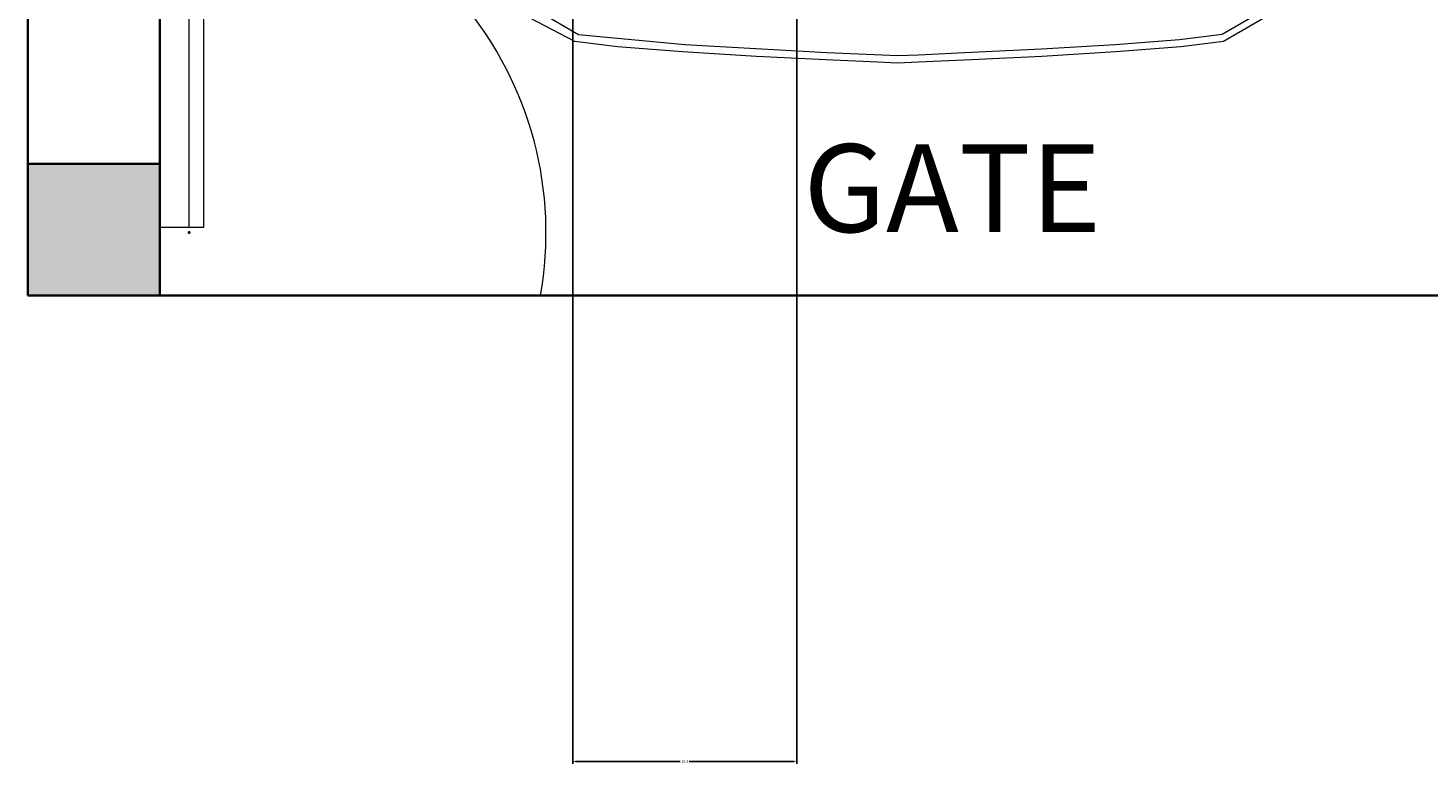
# Model space of a CAD drawing. Units: inches. Extents: x 5 to 421, y -617 to 43.
# Tile 1 of 15: x 37 to 133, y -617 to -566. Entities that reach past the tile are written whole.
import ezdxf

# ---------------------------------------------------------------- set-up
doc = ezdxf.new("R2010")
doc.units = ezdxf.units.IN
doc.header["$MEASUREMENT"] = 0
for name, color, linetype, lineweight in [('A-ANNO-DIMS', 2, 'Continuous', 18), ('A-ANNO-TEXT', 7, 'Continuous', 18), ('A-SITE-GATE', 3, 'Continuous', 20), ('A-SITE-VEHC', 8, 'Continuous', 13), ('A-WALL', 7, 'Continuous', 35)]:
    doc.layers.add(name, color=color, linetype=linetype, lineweight=lineweight)
doc.layers.add('A-WALL-PATT', color=251, linetype='Continuous', lineweight=13, true_color=0x636466)
doc.styles.get("Standard").update_dxf_attribs({"font": 'arial.ttf'})
doc.dimstyles.get("Standard").update_dxf_attribs({"dimtxt": 0.18, "dimasz": 0.18, "dimexe": 0.18, "dimexo": 0.0625, "dimgap": 0.09, "dimtad": 0, "dimtih": 1, "dimtoh": 1, "dimdec": 0, "dimzin": 0, "dimdsep": 46, "dimlunit": 3, "dimtxsty": 'Standard', "dimcen": 0.09, "dimadec": 0, "dimazin": 0, "dimtfac": 1, "dimtdec": 0, "dimtofl": 0, "dimtmove": 0, "dimatfit": 3, "dimfxl": 1, "dimtolj": 1, "dimtzin": 0, "dimarcsym": 0})

# ---------------------------------------------------------------- blocks, each defined once
blk = doc.blocks.new('*D78')
at = {"layer": 'A-ANNO-DIMS', "color": 0, "lineweight": -2, "transparency": 16777216}
for p, q in [((74.624, -338.19), (74.624, -616.599)), ((89.924, -338.331), (89.924, -616.599)), ((74.804, -616.419), (81.958, -616.419)), ((89.744, -616.419), (82.589, -616.419))]:
    blk.add_line(p, q, dxfattribs=at)
at = {"layer": 'A-ANNO-DIMS', "color": 0, "transparency": 16777216}
for points in [[(74.804, -616.389), (74.804, -616.449), (74.624, -616.419)], [(89.744, -616.389), (89.744, -616.449), (89.924, -616.419)]]:
    blk.add_solid(points, dxfattribs=at)
at = {"layer": 'Defpoints', "color": 0, "transparency": 16777216}
for p in [(74.624, -338.127), (89.924, -338.269), (89.924, -616.419)]:
    blk.add_point(p, dxfattribs=at)
at = {"layer": 'A-ANNO-DIMS', "color": 0, "transparency": 16777216, "insert": (82.274, -616.419), "char_height": 0.18, "attachment_point": 5}
blk.add_mtext('\\A1;15.3', dxfattribs=at)
blk = doc.blocks.new('*D81')
at = {"layer": 'A-ANNO-DIMS', "color": 0, "lineweight": -2, "transparency": 16777216}
for p, q in [((78.334, -555.287), (67.254, -564.56)), ((78.514, -555.287), (78.334, -555.287)), ((48.33, -580.324), (48.51, -580.324)), ((48.42, -580.414), (48.42, -580.234))]:
    blk.add_line(p, q, dxfattribs=at)
at = {"layer": 'A-ANNO-DIMS', "color": 0, "transparency": 16777216}
blk.add_solid([(67.235, -564.537), (67.274, -564.583), (67.116, -564.676)], dxfattribs=at)
at = {"layer": 'Defpoints', "color": 0, "transparency": 16777216}
for p in [(67.116, -564.676), (48.42, -580.324)]:
    blk.add_point(p, dxfattribs=at)
at = {"layer": 'A-ANNO-DIMS', "color": 0, "transparency": 16777216, "insert": (78.994, -555.287), "char_height": 0.18, "attachment_point": 5}
blk.add_mtext('\\A1;R24.38', dxfattribs=at)
blk = doc.blocks.new('*D82')
at = {"layer": 'A-ANNO-DIMS', "color": 0, "lineweight": -2, "transparency": 16777216}
for p, q in [((128.083, -555.094), (128.263, -555.094)), ((128.263, -555.094), (139.433, -564.316)), ((158.33, -579.992), (158.51, -579.992)), ((158.42, -580.082), (158.42, -579.902))]:
    blk.add_line(p, q, dxfattribs=at)
at = {"layer": 'A-ANNO-DIMS', "color": 0, "transparency": 16777216}
blk.add_solid([(139.452, -564.293), (139.414, -564.339), (139.572, -564.431)], dxfattribs=at)
at = {"layer": 'Defpoints', "color": 0, "transparency": 16777216}
for p in [(139.572, -564.431), (158.42, -579.992)]:
    blk.add_point(p, dxfattribs=at)
at = {"layer": 'A-ANNO-DIMS', "color": 0, "transparency": 16777216, "insert": (127.603, -555.094), "char_height": 0.18, "attachment_point": 5}
blk.add_mtext('\\A1;R24.44', dxfattribs=at)

msp = doc.modelspace()

# ---------------------------------------------------------------- hatches: boundary and pattern name
at = {"layer": 'A-WALL-PATT'}
h = msp.add_hatch(color=256, dxfattribs=at)
h.dxf.hatch_style = 1
h.paths.add_polyline_path([(46.4196, -88.1188), (37.4196, -88.1188), (37.4196, -166.6119), (46.4196, -166.6119), (46.4196, -122.6188), (135.4196, -122.6188), (135.4196, -120.3688), (135.4196, -118.1188), (46.4196, -118.1188)])
h.paths.add_polyline_path([(82.4196, 10.8812), (37.4196, 10.8812), (37.4196, -28.1188), (46.4196, -28.1188), (46.4196, 1.8812), (82.4196, 1.8812)])
h.paths.add_polyline_path([(215.5968, 10.8812), (142.4196, 10.8812), (142.4196, 1.8812), (178.4196, 1.8812), (178.4196, -118.1188), (175.4196, -118.1188), (175.4196, -122.6188), (182.9196, -122.6188), (182.9196, -80.6188), (211.9196, -80.6188), (211.9196, -78.3688), (211.9196, -76.1188), (182.9196, -76.1188), (182.9196, 1.8812), (215.5968, 1.8812)])
h.paths.add_polyline_path([(274.4196, 10.8812), (239.5968, 10.8812), (239.5968, 1.8812), (242.9196, 1.8812), (242.9196, -76.1188), (239.9196, -76.1188), (239.9196, -80.6188), (242.9196, -80.6188), (242.9196, -83.6188), (247.4196, -83.6188), (247.4196, 1.8812), (274.4196, 1.8812)])
h.paths.add_polyline_path([(370.4196, 10.8812), (334.4196, 10.8812), (334.4196, 1.8812), (361.4196, 1.8812), (361.4196, -28.1188), (370.4196, -28.1188)])
h.paths.add_polyline_path([(370.4196, -88.1188), (361.4196, -88.1188), (361.4196, -118.1188), (247.4196, -118.1188), (247.4196, -115.1188), (242.9196, -115.1188), (242.9196, -118.1188), (220.4196, -118.1188), (220.4196, -158.6188), (224.9196, -158.6188), (224.9196, -122.6188), (326.9196, -122.6188), (326.9196, -170.7662), (331.4196, -170.7662), (331.4196, -122.6188), (370.4196, -122.6188)])
h.paths.add_polyline_path([(388.4196, -122.6188), (388.4196, -118.1188), (379.4196, -118.1188), (379.4196, -122.6188), (379.4196, -154.8688), (388.4196, -154.8688)])
h.paths.add_polyline_path([(388.4196, -214.8688), (379.4196, -214.8688), (379.4196, -247.1188), (388.4196, -247.1188)])
h.paths.add_polyline_path([(371.0265, -242.6188), (331.4196, -242.6188), (331.4196, -239.6188), (326.9196, -239.6188), (326.9196, -242.6188), (224.9196, -242.6188), (224.9196, -206.6188), (220.4196, -206.6188), (220.4196, -343.6188), (224.9196, -343.6188), (229.4196, -343.6188), (229.4196, -247.1188), (261.5265, -247.1188), (261.5265, -276.1188), (263.7765, -276.1188), (266.0265, -276.1188), (266.0265, -247.1188), (362.0265, -247.1188), (362.0265, -265.1188), (371.0265, -265.1188), (371.0265, -247.1188)])
h.paths.add_polyline_path([(371.0265, -289.1188), (362.0265, -289.1188), (362.0265, -307.1188), (266.0265, -307.1188), (266.0265, -304.1188), (261.5265, -304.1188), (261.5265, -307.1188), (261.5265, -311.6188), (362.0265, -311.6188), (362.0265, -353.6188), (371.0265, -353.6188)])
h.paths.add_polyline_path([(371.0265, -413.6188), (362.0265, -413.6188), (362.0265, -455.6188), (325.7231, -455.6188), (325.7231, -464.6188), (361.4196, -464.6188), (371.0265, -464.6188)])
h.paths.add_polyline_path([(265.7231, -455.6188), (229.4196, -455.6188), (229.4196, -383.6188), (220.4196, -383.6188), (220.4196, -386.6188), (207.4649, -386.6188), (207.4649, -395.6188), (220.4196, -395.6188), (220.4196, -455.6188), (216.0568, -455.6188), (216.0568, -464.6188), (265.7231, -464.6188)])
h.paths.add_polyline_path([(169.4196, -386.6188), (137.9196, -386.6188), (137.9196, -395.6188), (160.4196, -395.6188), (160.4196, -424.2032), (169.4196, -424.2032)])
h.paths.add_polyline_path([(169.4196, -453.7423), (160.4196, -453.7423), (160.4196, -464.6188), (169.4196, -464.6188)])
h.paths.add_polyline_path([(46.4196, -575.6188), (37.4196, -575.6188), (37.4196, -584.6188), (46.4196, -584.6188)])
h.paths.add_polyline_path([(169.4196, -575.6188), (160.4196, -575.6188), (160.4196, -579.5504), (160.4196, -584.6188), (169.4196, -584.6188)])
h.paths.add_polyline_path([(46.4196, -226.6119), (37.4196, -226.6119), (37.4196, -292.8008), (46.4196, -292.8008)])
h.paths.add_polyline_path([(46.4196, -352.8008), (37.4196, -352.8008), (37.4196, -395.6188), (77.9196, -395.6188), (77.9196, -386.6188), (46.4196, -386.6188)])

# ---------------------------------------------------------------- linework, layer by layer
at = {"layer": 'A-SITE-GATE'}
for p, q in [((48.4196, -579.9431), (48.4196, -555.9431)), ((49.4196, -579.9431), (49.4196, -555.9431)), ((46.4196, -579.9431), (49.4196, -579.9431))]:
    msp.add_line(p, q, dxfattribs=at)
msp.add_arc((48.4196, -580.3243), 24.3812, 349.855002, 90, dxfattribs=at)
at = {"layer": 'A-SITE-VEHC'}
for p, q in [((74.7792, -567.2796), (71.7198, -565.6789)), ((72.2382, -565.178), (75.0189, -566.7885)), ((118.974, -566.7678), (121.7446, -565.1852)), ((122.0961, -565.5274), (119.0765, -567.2796)), ((75.0189, -566.7885), (82.2894, -567.4867)), ((116.0787, -567.1303), (118.974, -566.7678)), ((77.6917, -567.6453), (74.7792, -567.2796)), ((82.1333, -567.9907), (77.6917, -567.6453)), ((87.1858, -568.2946), (82.1333, -567.9907)), ((82.2894, -567.4867), (91.9744, -568.0197)), ((101.8586, -568.0147), (106.6413, -567.7735)), ((106.6413, -567.7735), (111.6636, -567.472)), ((111.7222, -567.9907), (106.6696, -568.2946)), ((111.6636, -567.472), (116.0787, -567.1303)), ((116.1638, -567.6453), (111.7222, -567.9907)), ((119.0765, -567.2796), (116.1638, -567.6453)), ((91.9189, -568.5363), (87.1858, -568.2946)), ((95.4303, -568.6963), (91.9189, -568.5363)), ((91.9744, -568.0197), (96.8252, -568.2322)), ((96.8041, -568.7543), (95.4303, -568.6963)), ((98.2421, -568.6963), (96.8041, -568.7543)), ((96.8252, -568.2322), (98.2512, -568.1745)), ((101.8724, -568.5363), (98.2421, -568.6963)), ((98.2512, -568.1745), (101.8586, -568.0147)), ((106.6696, -568.2946), (101.8724, -568.5363))]:
    msp.add_line(p, q, dxfattribs=at)
at = {"layer": 'A-WALL'}
for p, q in [((37.4196, 10.8812), (37.4196, -584.6188)), ((46.4196, -395.6188), (46.4196, -584.6188)), ((37.4196, -575.6188), (46.4196, -575.6188)), ((37.4196, -584.6188), (169.4196, -584.6188))]:
    msp.add_line(p, q, dxfattribs=at)

# ---------------------------------------------------------------- texts
at = {"layer": 'A-ANNO-TEXT', "insert": (90.3829, -574.2867), "char_height": 6, "attachment_point": 1}
msp.add_mtext('GATE', dxfattribs=at)

# ---------------------------------------------------------------- dimensions: what is measured, and where the dimension line sits
at = {"layer": 'A-ANNO-DIMS'}
dim = msp.add_linear_dim(base=(89.9238, -616.4188), p1=(74.6237, -338.1275), p2=(89.9238, -338.2687), dimstyle='Standard', override={"dimdec": 1, "dimlfac": 1, "dimrnd": 0, "dimzin": 0, "dimdsep": 46, "dimlunit": 2}, dxfattribs=at)
dim.commit()
dim.dimension.update_dxf_attribs({"geometry": '*D78', "text_midpoint": (82.2737, -616.4188)})
for center, mpoint, picture, middle in [((48.4196, -580.3243), (67.1163, -564.6758), '*D81', (78.9943, -555.2866)), ((158.4196, -579.9922), (139.5717, -564.4307), '*D82', (127.6034, -555.0938))]:
    dim = msp.add_radius_dim(center=center, mpoint=mpoint, dimstyle='Standard', override={"dimdec": 2, "dimlfac": 1, "dimrnd": 0, "dimzin": 0, "dimdsep": 46, "dimlunit": 2}, dxfattribs=at)
    dim.commit()
    dim.dimension.update_dxf_attribs({"geometry": picture, "text_midpoint": middle, "dimtype": 164})

doc.saveas('drawing.dxf')
